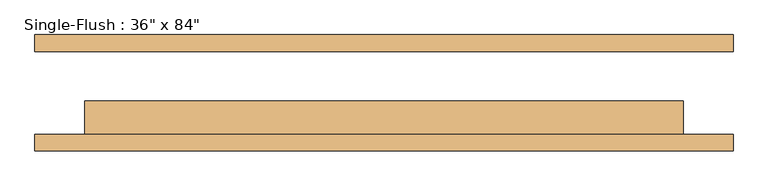
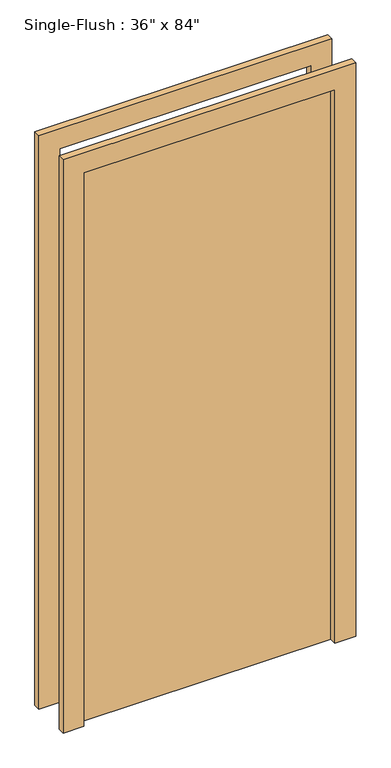
"""IFC4 building model written with IfcOpenShell, lengths in millimetres: door geometry."""

from ifc_helpers import new_model, si_unit, frame, origin, origin_with_axes, place, context, project, spatial, polyline, outline, extrude, source, transform, mapped, element, save


def door_a3eb833a(model_context):
    return source(origin(), model_context, "Body", "SweptSolid", [
        extrude(outline(polyline([(2209.8, -533.4), (0.0, -533.4), (0.0, -457.2), (2133.6, -457.2), (2133.6, 457.2), (0.0, 457.2), (0.0, 533.4), (2209.8, 533.4), (2209.8, -533.4)])), frame((0.0, -88.9, 0.0), z_axis=(0.0, 1.0, 0.0), x_axis=(0.0, 0.0, 1.0)), (0.0, 0.0, 1.0), 25.4),
        extrude(outline(polyline([(2209.8, 533.4), (2209.8, -533.4), (0.0, -533.4), (0.0, -457.2), (2133.6, -457.2), (2133.6, 457.2), (0.0, 457.2), (0.0, 533.4), (2209.8, 533.4)])), frame((0.0, 63.5, 0.0), z_axis=(0.0, 1.0, 0.0), x_axis=(0.0, 0.0, 1.0)), (0.0, 0.0, 1.0), 25.4),
        extrude(outline(polyline([(457.2, -12.7), (457.2, -63.5), (-457.2, -63.5), (-457.2, -12.7), (457.2, -12.7)])), origin_with_axes(), (0.0, 0.0, 1.0), 2133.6),
    ])


if __name__ == "__main__":
    model = new_model("IFC4")
    model_context = context("Model", 3, world=origin())
    ifc_project = project(units=[si_unit("LENGTHUNIT", "METRE", prefix="MILLI")], contexts=[model_context])
    site = spatial("IfcSite", under=ifc_project)
    building = spatial("IfcBuilding", under=site)
    placement = place(None, origin())
    door_shape = door_a3eb833a(model_context)
    element("IfcDoor", 1, ObjectType="Single-Flush : 36\" x 84\"", at=placement, inside=building, context=model_context, shape_type="MappedRepresentation", body=[
        mapped(door_shape, transform((0.0, 0.0, 0.0), x_axis=(1.0, 0.0, 0.0), y_axis=(0.0, 1.0, 0.0), z_axis=(0.0, 0.0, 1.0))),
    ])
    save(model, "model.ifc")

# Revit data of these elements
# Type "Single-Flush : 36\" x 84\""
#   Type Mark = "1"
#   Assembly Code = "C1020"
#   Thickness = 0' - 2"
#   Height = 7' - 0"
#   Trim Projection Ext = 0' - 1"
#   Trim Projection Int = 0' - 1"
#   Trim Width = 0' - 3"
#   Width = 3' - 0"
#   Door Material = Door - Panel
#   Frame Material = Door - Frame
#   Function = (empty or 0)
#   Wall Closure = (empty or 0)
# Element 1 (IfcDoor, "Single-Flush : 36\" x 84\"")
#   Materials on its faces: "Door - Frame", "Door - Panel"
# Materials
#   "Door - Panel": class "Wood", colour RGB 114 82 51, transparency 0
#   "Door - Frame": colour RGB 153 76 43, transparency 0
